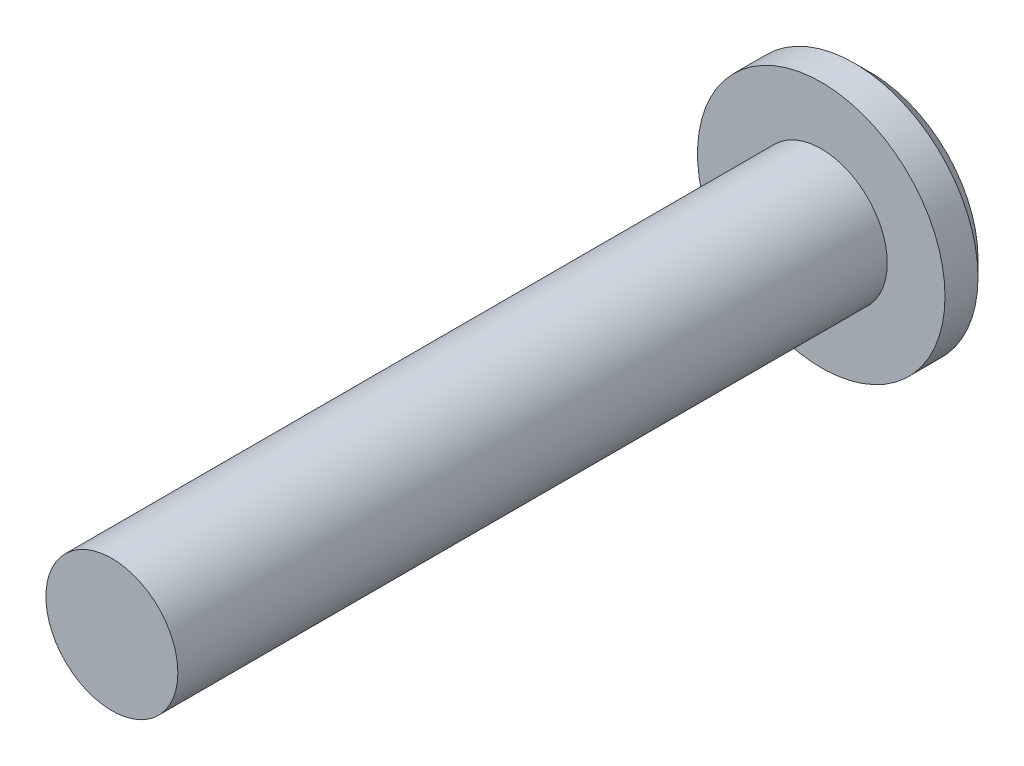
from build123d import *

# Parameters (mm, degrees)
HEAD_PROFILE_15_R      = 7.5
HEAD_15X3_DEPTH        = 3
SHANK_PROFILE_8_R      = 4
SHANK_8X43_DEPTH       = 43
HEAD_CHAMFER_1X45_SIZE = 1


with BuildPart() as part:
    # Head Profile Ø15 → Head Ø15x3 (new body)
    with BuildSketch(Plane.XY):
        Circle(HEAD_PROFILE_15_R)
    extrude(amount=HEAD_15X3_DEPTH)

    # Shank Profile Ø8 → Shank Ø8x43 (add)
    with BuildSketch(Plane.XY.offset(3)):
        Circle(SHANK_PROFILE_8_R)
    extrude(amount=SHANK_8X43_DEPTH)

    # Head Chamfer 1x45°
    head_chamfer_1x45_edges = [part.edges().sort_by_distance(p)[0] for p in [
        (-7.5, 0, 0),
    ]]
    chamfer(head_chamfer_1x45_edges, length=HEAD_CHAMFER_1X45_SIZE)


solid = part.part
